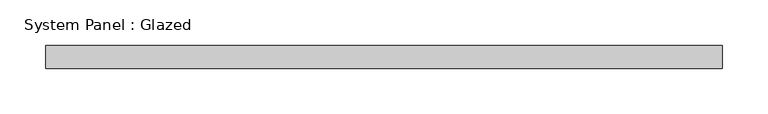
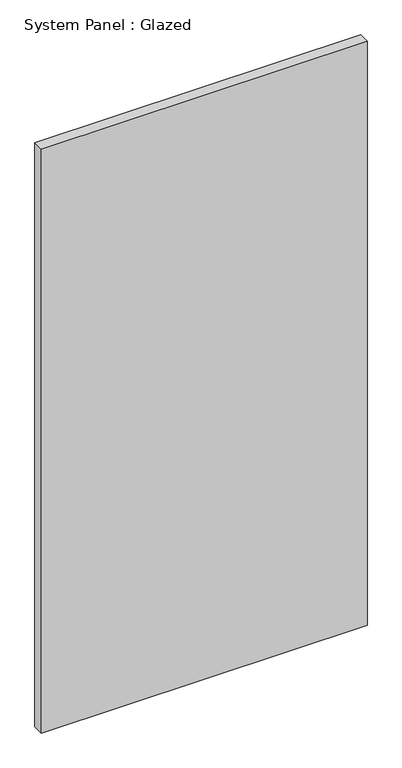
"""IFC4 building model written with IfcOpenShell, lengths in millimetres: plate geometry, System Panel : Glazed."""

from ifc_helpers import new_model, si_unit, origin, origin_with_axes, place, context, project, spatial, polyline, outline, extrude, source, transform, mapped, element, save


def system_panel_glazed_b08c4d22(model_context):
    return source(origin(), model_context, "Body", "SweptSolid", [
        extrude(outline(polyline([(371.475, 19.05), (-371.475, 19.05), (-371.475, 44.45), (371.475, 44.45), (371.475, 19.05)])), origin_with_axes(), (0.0, 0.0, 1.0), 1408.0629342),
    ])


if __name__ == "__main__":
    model = new_model("IFC4")
    model_context = context("Model", 3, world=origin())
    ifc_project = project(units=[si_unit("LENGTHUNIT", "METRE", prefix="MILLI")], contexts=[model_context])
    site = spatial("IfcSite", under=ifc_project)
    building = spatial("IfcBuilding", under=site)
    placement = place(None, origin())
    system_panel_glazed_shape = system_panel_glazed_b08c4d22(model_context)
    element("IfcPlate", 1, ObjectType="System Panel : Glazed", at=placement, inside=building, context=model_context, shape_type="MappedRepresentation", body=[
        mapped(system_panel_glazed_shape, transform((0.0, 0.0, 0.0), x_axis=(1.0, 0.0, 0.0), y_axis=(0.0, 1.0, 0.0), z_axis=(0.0, 0.0, 1.0))),
    ])
    save(model, "model.ifc")

# Revit data of these elements
# Type "System Panel : Glazed"
#   Construction Type Id = "GSP4R"
#   Analytic Construction = "1/8 in Pilkington single glazing"
#   Visual Light Transmittance = 0.9
#   Solar Heat Gain Coefficient = 0.86
#   Heat Transfer Coefficient (U) = 1.18115 BTU/(h·ft²·°F)
#   Define Thermal Properties by = 1
# Element 1 (IfcPlate, "System Panel : Glazed")
#   Materials on its faces: "Glass"
# Materials
#   "Glass": class "Glass", colour RGB 0 128 192, transparency 0.75, Description = "Soda Lime Glass", Cost = 0
